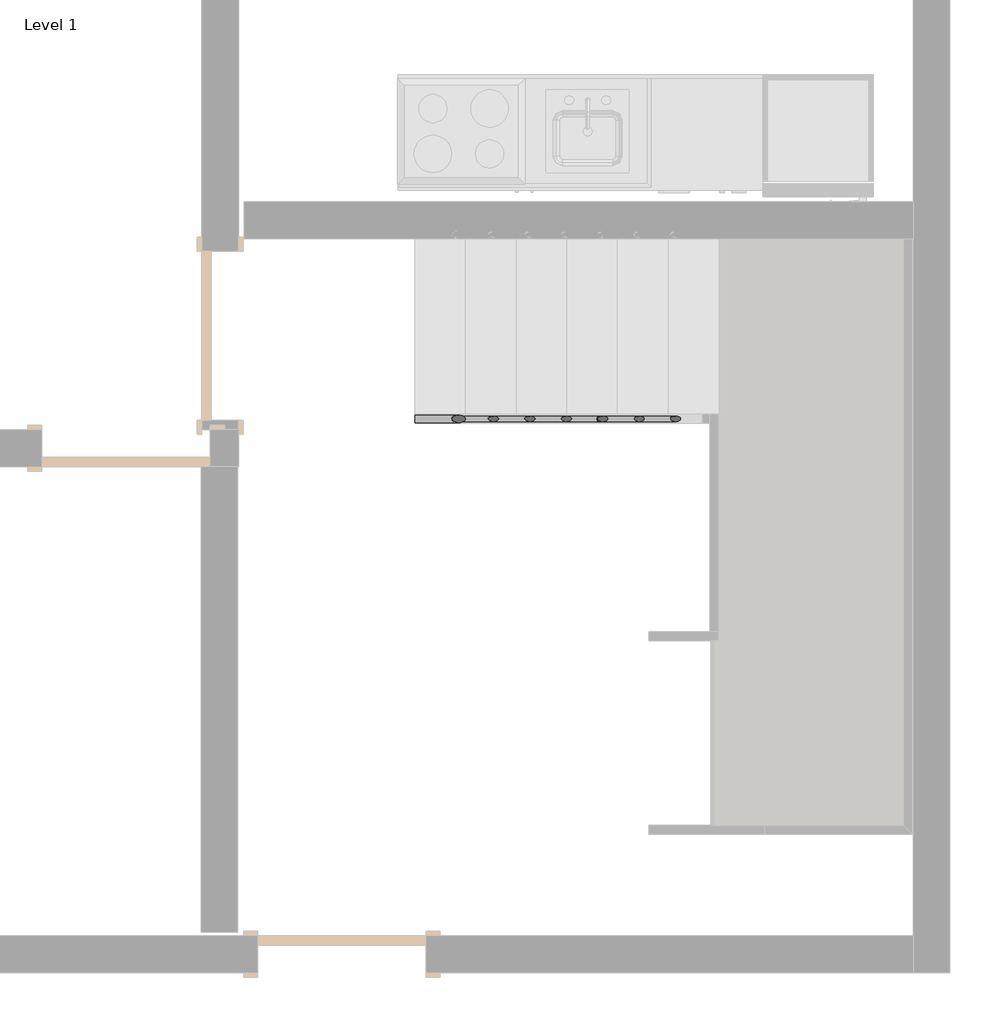
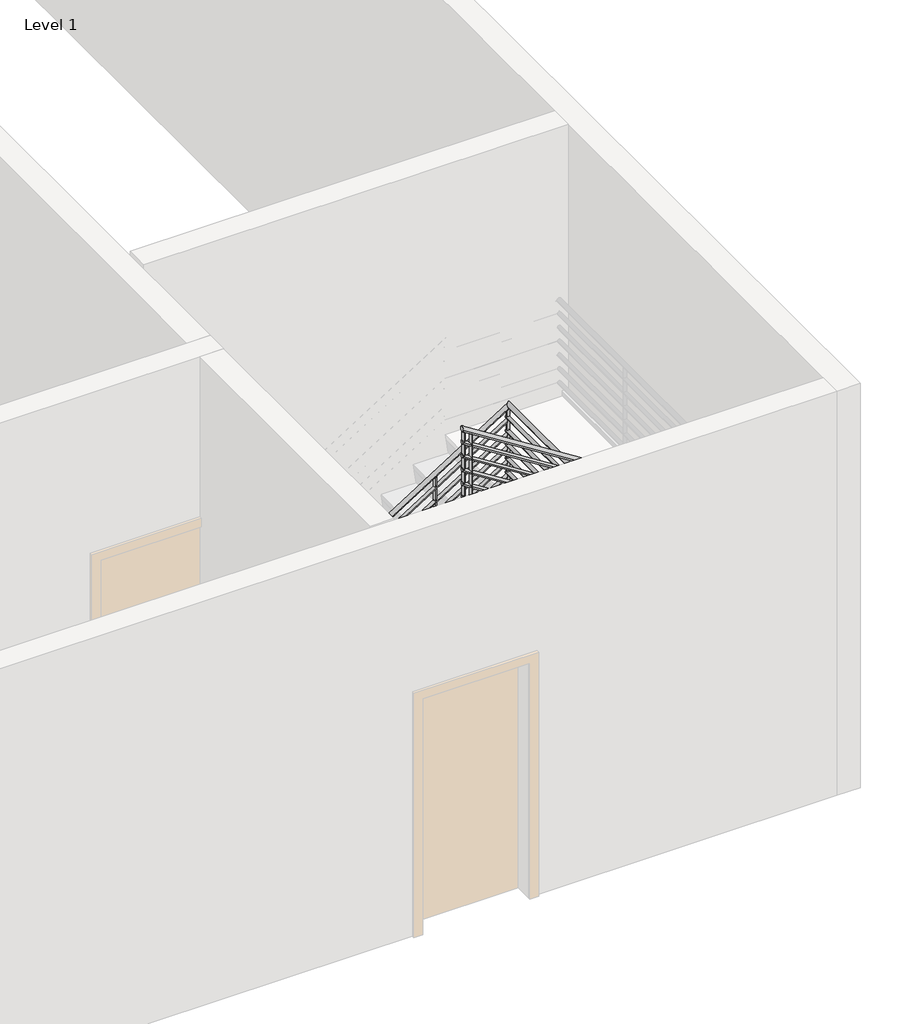
# One storey, part 2 of 4: 1 railing.
"""IFC4 building model written with IfcOpenShell, lengths in millimetres."""

from ifc_helpers import new_model, si_unit, point, frame, frame_2d, origin, place, context, project, spatial, circle_curve, ellipse_curve, trimmed, segment, composite_curve, outline, extrude, element, save
from ifc_brep_helpers import plane_surface, cylinder_surface, advanced_brep

model = new_model("IFC4")

# Units and contexts
model_context = context("Model", 3, world=origin())
ifc_project = project(units=[si_unit("LENGTHUNIT", "METRE", prefix="MILLI")], contexts=[model_context])

# Site, building, storey
site = spatial("IfcSite", under=ifc_project)
building = spatial("IfcBuilding", under=site)
storey = spatial("IfcBuildingStorey", under=building, Name="Level 1", Elevation=0.0)

# Railing
placement = place(None, origin())
element("IfcRailing", 1, ObjectType="900mm Pipe", at=placement, inside=storey, context=model_context, shape_type="SolidModel", body=[
    advanced_brep(
    [(-8739.5726707, 1114.9053702, 1050.2491997), (-8739.5726707, 1154.9053702, 1050.2491997), (-7121.1861826, 1114.9053702, 2073.7347258), (-7087.3793333, 1154.9053702, 2095.1145514)],
    [
        (0, 1, ellipse_curve(frame((-8739.5726707, 1134.9053702, 1050.2491997), z_axis=(-1.0, 0.0, 0.0), x_axis=(0.0, 0.0, -1.0)), 23.6638438, 20.0)),
        (1, 0, ellipse_curve(frame((-8739.5726707, 1134.9053702, 1050.2491997), z_axis=(-1.0, 0.0, 0.0), x_axis=(0.0, 0.0, -1.0)), 23.6638438, 20.0)),
        (2, 3, ellipse_curve(frame((-7104.2827579, 1134.9053702, 2084.4246386), z_axis=(0.5976263089853383, -0.7071067811865501, 0.37794549184843773), x_axis=(-0.5976263089853444, -0.7071067811865451, -0.37794549184843684)), 28.2842712, 20.0)),
        (3, 2, ellipse_curve(frame((-7104.2827579, 1134.9053702, 2084.4246386), z_axis=(0.5976263089853383, -0.7071067811865501, 0.37794549184843773), x_axis=(-0.5976263089853444, -0.7071067811865451, -0.37794549184843684)), 28.2842712, 20.0)),
        (0, 2),
        (3, 1),
    ],
    [
        plane_surface(frame((-8739.5726707, 1134.9053702, 1073.9130435), z_axis=(-1.0, 0.0, 0.0), x_axis=(0.0, 1.0, 0.0))),
        plane_surface(frame((-7114.9726707, 1134.9053702, 2101.3280632), z_axis=(0.5976263089853383, -0.7071067811865501, 0.37794549184843773), x_axis=(0.80177477810702, 0.527062745346942, -0.28171273961037624))),
        cylinder_surface(frame((-8728.8827579, 1134.9053702, 1057.0096189), z_axis=(-0.8451712313980437, 0.0, -0.5344956404098301), x_axis=(0.0, 1.0, 0.0)), 20.0),
    ],
    [
        (0, [[1, 2]]),
        (1, [[3, 4]]),
        (2, [[-1, 5, -4, 6]]),
        (2, [[-2, -6, -3, -5]]),
    ],
),
    advanced_brep(
    [(-7134.9726707, 1107.3120327, 2097.3913043), (-7094.9726707, 1141.118882, 2097.3913043), (-7134.9726707, -43.6804955, 2097.3913043), (-7094.9726707, -43.6804955, 2097.3913043)],
    [
        (0, 1, ellipse_curve(frame((-7114.9726707, 1124.2154574, 2097.3913043), z_axis=(-0.5976263089853383, 0.7071067811865501, -0.37794549184843773), x_axis=(0.5976263089853447, 0.7071067811865448, 0.3779454918484371)), 28.2842712, 20.0)),
        (1, 0, ellipse_curve(frame((-7114.9726707, 1124.2154574, 2097.3913043), z_axis=(-0.5976263089853383, 0.7071067811865501, -0.37794549184843773), x_axis=(0.5976263089853447, 0.7071067811865448, 0.3779454918484371)), 28.2842712, 20.0)),
        (2, 3, ellipse_curve(frame((-7114.9726707, -43.6804955, 2097.3913043), z_axis=(0.0, -0.7071067811865477, 0.7071067811865474), x_axis=(0.0, 0.7071067811865474, 0.7071067811865477)), 28.2842712, 20.0)),
        (3, 2, ellipse_curve(frame((-7114.9726707, -43.6804955, 2097.3913043), z_axis=(0.0, -0.7071067811865477, 0.7071067811865474), x_axis=(0.0, 0.7071067811865474, 0.7071067811865477)), 28.2842712, 20.0)),
        (0, 2),
        (3, 1),
    ],
    [
        plane_surface(frame((-7114.9726707, 1134.9053702, 2117.3913043), z_axis=(-0.5976263089853383, 0.7071067811865501, -0.37794549184843773), x_axis=(0.80177477810702, 0.527062745346942, -0.28171273961037624))),
        plane_surface(frame((-7114.9726707, -23.6804955, 2117.3913043), z_axis=(0.0, -0.7071067811865477, 0.7071067811865474), x_axis=(1.0, 0.0, 0.0))),
        cylinder_surface(frame((-7114.9726707, 1134.9053702, 2097.3913043), z_axis=(0.0, 1.0, 0.0), x_axis=(1.0, 0.0, 0.0)), 20.0),
    ],
    [
        (0, [[1, 2]]),
        (1, [[3, 4]]),
        (2, [[-1, 5, -4, 6]]),
        (2, [[-2, -6, -3, -5]]),
    ],
),
    advanced_brep(
    [(-7114.9726707, -23.6804955, 2283.7037451), (-7114.9726707, -63.6804955, 2283.7037451), (-8189.5726707, -23.6804955, 2963.2926779), (-8189.5726707, -63.6804955, 2963.2926779)],
    [
        (0, 1, ellipse_curve(frame((-7114.9726707, -43.6804955, 2283.7037451), z_axis=(0.4824439654458172, 0.0, -0.8759268349610687), x_axis=(0.8759268349610684, 0.0, 0.48244396544581747)), 22.8329573, 20.0)),
        (1, 0, ellipse_curve(frame((-7114.9726707, -43.6804955, 2283.7037451), z_axis=(0.4824439654458172, 0.0, -0.8759268349610687), x_axis=(0.8759268349610684, 0.0, 0.48244396544581747)), 22.8329573, 20.0)),
        (2, 3, ellipse_curve(frame((-8189.5726707, -43.6804955, 2963.2926779), z_axis=(-1.0, 0.0, 0.0), x_axis=(0.0, 0.0, -1.0)), 23.6638438, 20.0)),
        (3, 2, ellipse_curve(frame((-8189.5726707, -43.6804955, 2963.2926779), z_axis=(-1.0, 0.0, 0.0), x_axis=(0.0, 0.0, -1.0)), 23.6638438, 20.0)),
        (0, 2),
        (3, 1),
    ],
    [
        plane_surface(frame((-7094.9726707, -43.6804955, 2294.7193676), z_axis=(0.4824439654458172, 0.0, -0.8759268349610687), x_axis=(0.8759268349610687, 0.0, 0.4824439654458172))),
        plane_surface(frame((-8189.5726707, -43.6804955, 2986.9565217), z_axis=(-1.0, 0.0, 0.0), x_axis=(0.0, -1.0, 0.0))),
        cylinder_surface(frame((-7105.6625835, -43.6804955, 2277.815943), z_axis=(0.8451712313980436, 0.0, -0.5344956404098304), x_axis=(0.0, -1.0, 0.0)), 20.0),
    ],
    [
        (0, [[1, 2]]),
        (1, [[3, 4]]),
        (2, [[-1, 5, -4, 6]]),
        (2, [[-2, -6, -3, -5]]),
    ],
),
    advanced_brep(
    [(-7134.9726707, -43.6804955, 2097.3913043), (-7094.9726707, -43.6804955, 2097.3913043), (-7134.9726707, -43.6804955, 2272.6881227), (-7094.9726707, -43.6804955, 2294.7193676)],
    [
        (0, 1, ellipse_curve(frame((-7114.9726707, -43.6804955, 2097.3913043), z_axis=(0.0, 0.7071067811865477, -0.7071067811865474), x_axis=(0.0, -0.7071067811865474, -0.7071067811865478)), 28.2842712, 20.0)),
        (1, 0, ellipse_curve(frame((-7114.9726707, -43.6804955, 2097.3913043), z_axis=(0.0, 0.7071067811865477, -0.7071067811865474), x_axis=(0.0, -0.7071067811865474, -0.7071067811865478)), 28.2842712, 20.0)),
        (2, 3, ellipse_curve(frame((-7114.9726707, -43.6804955, 2283.7037451), z_axis=(-0.4824439654458172, 0.0, 0.8759268349610687), x_axis=(-0.8759268349610689, 0.0, -0.4824439654458169)), 22.8329573, 20.0)),
        (3, 2, ellipse_curve(frame((-7114.9726707, -43.6804955, 2283.7037451), z_axis=(-0.4824439654458172, 0.0, 0.8759268349610687), x_axis=(-0.8759268349610689, 0.0, -0.4824439654458169)), 22.8329573, 20.0)),
        (0, 2),
        (3, 1),
    ],
    [
        plane_surface(frame((-7114.9726707, -43.6804955, 2097.3913043), z_axis=(0.0, 0.7071067811865477, -0.7071067811865474), x_axis=(1.0, 0.0, 0.0))),
        plane_surface(frame((-7114.9726707, -43.6804955, 2283.7037451), z_axis=(-0.4824439654458172, 0.0, 0.8759268349610687), x_axis=(0.8759268349610687, 0.0, 0.4824439654458172))),
        cylinder_surface(frame((-7114.9726707, -43.6804955, 2097.3913043), z_axis=(0.0, 0.0, -1.0), x_axis=(1.0, 0.0, 0.0)), 20.0),
    ],
    [
        (0, [[1, 2]]),
        (1, [[3, 4]]),
        (2, [[-1, 5, -4, 6]]),
        (2, [[-2, -6, -3, -5]]),
    ],
),
    advanced_brep(
    [(-8739.5726707, 1119.9053702, 931.1651606), (-8739.5726707, 1149.9053702, 931.1651606), (-7129.9726707, 1119.9053702, 1949.0940144), (-7129.9726707, 1149.9053702, 1949.0940144)],
    [
        (0, 1, ellipse_curve(frame((-8739.5726707, 1134.9053702, 931.1651606), z_axis=(-1.0, 0.0, 0.0), x_axis=(0.0, 0.0, -1.0)), 17.7478828, 15.0)),
        (1, 0, ellipse_curve(frame((-8739.5726707, 1134.9053702, 931.1651606), z_axis=(-1.0, 0.0, 0.0), x_axis=(0.0, 0.0, -1.0)), 17.7478828, 15.0)),
        (2, 3, ellipse_curve(frame((-7129.9726707, 1134.9053702, 1949.0940144), z_axis=(1.0, 0.0, 0.0), x_axis=(0.0, 0.0, -1.0)), 17.7478828, 15.0)),
        (3, 2, ellipse_curve(frame((-7129.9726707, 1134.9053702, 1949.0940144), z_axis=(1.0, 0.0, 0.0), x_axis=(0.0, 0.0, -1.0)), 17.7478828, 15.0)),
        (1, 3),
        (2, 0),
    ],
    [
        plane_surface(frame((-8739.5726707, 1134.9053702, 948.9130435), z_axis=(-1.0, 0.0, 0.0), x_axis=(0.0, 1.0, 0.0))),
        plane_surface(frame((-7129.9726707, 1134.9053702, 1966.8418972), z_axis=(1.0, 0.0, 0.0), x_axis=(0.0, 1.0, 0.0))),
        cylinder_surface(frame((-8731.5552361, 1134.9053702, 936.235475), z_axis=(-0.8451712313980437, 0.0, -0.5344956404098302), x_axis=(0.0, 1.0, 0.0)), 15.0),
    ],
    [
        (0, [[1, 2]]),
        (1, [[3, 4]]),
        (2, [[-2, 5, -3, 6]]),
        (2, [[-1, -6, -4, -5]]),
    ],
),
    advanced_brep(
    [(-7129.9726707, 1149.9053702, 1977.3913043), (-7099.9726707, 1149.9053702, 1977.3913043), (-7129.9726707, -28.6804955, 1977.3913043), (-7099.9726707, -28.6804955, 1977.3913043)],
    [
        (0, 1, circle_curve(frame((-7114.9726707, 1149.9053702, 1977.3913043), z_axis=(0.0, 1.0, 0.0), x_axis=(1.0, 0.0, 0.0)), 15.0)),
        (1, 0, circle_curve(frame((-7114.9726707, 1149.9053702, 1977.3913043), z_axis=(0.0, 1.0, 0.0), x_axis=(1.0, 0.0, 0.0)), 15.0)),
        (2, 3, circle_curve(frame((-7114.9726707, -28.6804955, 1977.3913043), z_axis=(0.0, -1.0, 0.0), x_axis=(1.0, 0.0, 0.0)), 15.0)),
        (3, 2, circle_curve(frame((-7114.9726707, -28.6804955, 1977.3913043), z_axis=(0.0, -1.0, 0.0), x_axis=(1.0, 0.0, 0.0)), 15.0)),
        (1, 3),
        (2, 0),
    ],
    [
        plane_surface(frame((-7114.9726707, 1149.9053702, 1992.3913043), z_axis=(0.0, 1.0, 0.0), x_axis=(0.0, 0.0, -1.0))),
        plane_surface(frame((-7114.9726707, -28.6804955, 1992.3913043), z_axis=(0.0, -1.0, 0.0), x_axis=(0.0, 0.0, -1.0))),
        cylinder_surface(frame((-7114.9726707, 1149.9053702, 1977.3913043), z_axis=(0.0, 1.0, 0.0), x_axis=(1.0, 0.0, 0.0)), 15.0),
    ],
    [
        (0, [[1, 2]]),
        (1, [[3, 4]]),
        (2, [[-2, 5, -3, 6]]),
        (2, [[-1, -6, -4, -5]]),
    ],
),
    advanced_brep(
    [(-7099.9726707, -28.6804955, 2155.1335401), (-7099.9726707, -58.6804955, 2155.1335401), (-8189.5726707, -28.6804955, 2844.2086389), (-8189.5726707, -58.6804955, 2844.2086389)],
    [
        (0, 1, ellipse_curve(frame((-7099.9726707, -43.6804955, 2155.1335401), z_axis=(1.0, 0.0, 0.0), x_axis=(0.0, 0.0, -1.0)), 17.7478828, 15.0)),
        (1, 0, ellipse_curve(frame((-7099.9726707, -43.6804955, 2155.1335401), z_axis=(1.0, 0.0, 0.0), x_axis=(0.0, 0.0, -1.0)), 17.7478828, 15.0)),
        (2, 3, ellipse_curve(frame((-8189.5726707, -43.6804955, 2844.2086389), z_axis=(-1.0, 0.0, 0.0), x_axis=(0.0, 0.0, -1.0)), 17.7478828, 15.0)),
        (3, 2, ellipse_curve(frame((-8189.5726707, -43.6804955, 2844.2086389), z_axis=(-1.0, 0.0, 0.0), x_axis=(0.0, 0.0, -1.0)), 17.7478828, 15.0)),
        (1, 3),
        (2, 0),
    ],
    [
        plane_surface(frame((-7099.9726707, -43.6804955, 2172.8814229), z_axis=(1.0, 0.0, 0.0), x_axis=(0.0, -1.0, 0.0))),
        plane_surface(frame((-8189.5726707, -43.6804955, 2861.9565217), z_axis=(-1.0, 0.0, 0.0), x_axis=(0.0, -1.0, 0.0))),
        cylinder_surface(frame((-7107.9901053, -43.6804955, 2160.2038545), z_axis=(0.8451712313980437, 0.0, -0.5344956404098303), x_axis=(0.0, -1.0, 0.0)), 15.0),
    ],
    [
        (0, [[1, 2]]),
        (1, [[3, 4]]),
        (2, [[-2, 5, -3, 6]]),
        (2, [[-1, -6, -4, -5]]),
    ],
),
    advanced_brep(
    [(-8739.5726707, 1119.9053702, 806.1651606), (-8739.5726707, 1149.9053702, 806.1651606), (-7129.9726707, 1119.9053702, 1824.0940144), (-7129.9726707, 1149.9053702, 1824.0940144)],
    [
        (0, 1, ellipse_curve(frame((-8739.5726707, 1134.9053702, 806.1651606), z_axis=(-1.0, 0.0, 0.0), x_axis=(0.0, 0.0, -1.0)), 17.7478828, 15.0)),
        (1, 0, ellipse_curve(frame((-8739.5726707, 1134.9053702, 806.1651606), z_axis=(-1.0, 0.0, 0.0), x_axis=(0.0, 0.0, -1.0)), 17.7478828, 15.0)),
        (2, 3, ellipse_curve(frame((-7129.9726707, 1134.9053702, 1824.0940144), z_axis=(1.0, 0.0, 0.0), x_axis=(0.0, 0.0, -1.0)), 17.7478828, 15.0)),
        (3, 2, ellipse_curve(frame((-7129.9726707, 1134.9053702, 1824.0940144), z_axis=(1.0, 0.0, 0.0), x_axis=(0.0, 0.0, -1.0)), 17.7478828, 15.0)),
        (1, 3),
        (2, 0),
    ],
    [
        plane_surface(frame((-8739.5726707, 1134.9053702, 823.9130435), z_axis=(-1.0, 0.0, 0.0), x_axis=(0.0, 1.0, 0.0))),
        plane_surface(frame((-7129.9726707, 1134.9053702, 1841.8418972), z_axis=(1.0, 0.0, 0.0), x_axis=(0.0, 1.0, 0.0))),
        cylinder_surface(frame((-8731.5552361, 1134.9053702, 811.235475), z_axis=(-0.8451712313980438, 0.0, -0.5344956404098301), x_axis=(0.0, 1.0, 0.0)), 15.0),
    ],
    [
        (0, [[1, 2]]),
        (1, [[3, 4]]),
        (2, [[-2, 5, -3, 6]]),
        (2, [[-1, -6, -4, -5]]),
    ],
),
    advanced_brep(
    [(-7129.9726707, 1149.9053702, 1852.3913043), (-7099.9726707, 1149.9053702, 1852.3913043), (-7129.9726707, -28.6804955, 1852.3913043), (-7099.9726707, -28.6804955, 1852.3913043)],
    [
        (0, 1, circle_curve(frame((-7114.9726707, 1149.9053702, 1852.3913043), z_axis=(0.0, 1.0, 0.0), x_axis=(1.0, 0.0, 0.0)), 15.0)),
        (1, 0, circle_curve(frame((-7114.9726707, 1149.9053702, 1852.3913043), z_axis=(0.0, 1.0, 0.0), x_axis=(1.0, 0.0, 0.0)), 15.0)),
        (2, 3, circle_curve(frame((-7114.9726707, -28.6804955, 1852.3913043), z_axis=(0.0, -1.0, 0.0), x_axis=(1.0, 0.0, 0.0)), 15.0)),
        (3, 2, circle_curve(frame((-7114.9726707, -28.6804955, 1852.3913043), z_axis=(0.0, -1.0, 0.0), x_axis=(1.0, 0.0, 0.0)), 15.0)),
        (1, 3),
        (2, 0),
    ],
    [
        plane_surface(frame((-7114.9726707, 1149.9053702, 1867.3913043), z_axis=(0.0, 1.0, 0.0), x_axis=(0.0, 0.0, -1.0))),
        plane_surface(frame((-7114.9726707, -28.6804955, 1867.3913043), z_axis=(0.0, -1.0, 0.0), x_axis=(0.0, 0.0, -1.0))),
        cylinder_surface(frame((-7114.9726707, 1149.9053702, 1852.3913043), z_axis=(0.0, 1.0, 0.0), x_axis=(1.0, 0.0, 0.0)), 15.0),
    ],
    [
        (0, [[1, 2]]),
        (1, [[3, 4]]),
        (2, [[-2, 5, -3, 6]]),
        (2, [[-1, -6, -4, -5]]),
    ],
),
    advanced_brep(
    [(-7099.9726707, -28.6804955, 2030.1335401), (-7099.9726707, -58.6804955, 2030.1335401), (-8189.5726707, -28.6804955, 2719.2086389), (-8189.5726707, -58.6804955, 2719.2086389)],
    [
        (0, 1, ellipse_curve(frame((-7099.9726707, -43.6804955, 2030.1335401), z_axis=(1.0, 0.0, 0.0), x_axis=(0.0, 0.0, -1.0)), 17.7478828, 15.0)),
        (1, 0, ellipse_curve(frame((-7099.9726707, -43.6804955, 2030.1335401), z_axis=(1.0, 0.0, 0.0), x_axis=(0.0, 0.0, -1.0)), 17.7478828, 15.0)),
        (2, 3, ellipse_curve(frame((-8189.5726707, -43.6804955, 2719.2086389), z_axis=(-1.0, 0.0, 0.0), x_axis=(0.0, 0.0, -1.0)), 17.7478828, 15.0)),
        (3, 2, ellipse_curve(frame((-8189.5726707, -43.6804955, 2719.2086389), z_axis=(-1.0, 0.0, 0.0), x_axis=(0.0, 0.0, -1.0)), 17.7478828, 15.0)),
        (1, 3),
        (2, 0),
    ],
    [
        plane_surface(frame((-7099.9726707, -43.6804955, 2047.8814229), z_axis=(1.0, 0.0, 0.0), x_axis=(0.0, -1.0, 0.0))),
        plane_surface(frame((-8189.5726707, -43.6804955, 2736.9565217), z_axis=(-1.0, 0.0, 0.0), x_axis=(0.0, -1.0, 0.0))),
        cylinder_surface(frame((-7107.9901053, -43.6804955, 2035.2038545), z_axis=(0.8451712313980436, 0.0, -0.5344956404098304), x_axis=(0.0, -1.0, 0.0)), 15.0),
    ],
    [
        (0, [[1, 2]]),
        (1, [[3, 4]]),
        (2, [[-2, 5, -3, 6]]),
        (2, [[-1, -6, -4, -5]]),
    ],
),
    advanced_brep(
    [(-8739.5726707, 1119.9053702, 681.1651606), (-8739.5726707, 1149.9053702, 681.1651606), (-7129.9726707, 1119.9053702, 1699.0940144), (-7129.9726707, 1149.9053702, 1699.0940144)],
    [
        (0, 1, ellipse_curve(frame((-8739.5726707, 1134.9053702, 681.1651606), z_axis=(-1.0, 0.0, 0.0), x_axis=(0.0, 0.0, -1.0)), 17.7478828, 15.0)),
        (1, 0, ellipse_curve(frame((-8739.5726707, 1134.9053702, 681.1651606), z_axis=(-1.0, 0.0, 0.0), x_axis=(0.0, 0.0, -1.0)), 17.7478828, 15.0)),
        (2, 3, ellipse_curve(frame((-7129.9726707, 1134.9053702, 1699.0940144), z_axis=(1.0, 0.0, 0.0), x_axis=(0.0, 0.0, -1.0)), 17.7478828, 15.0)),
        (3, 2, ellipse_curve(frame((-7129.9726707, 1134.9053702, 1699.0940144), z_axis=(1.0, 0.0, 0.0), x_axis=(0.0, 0.0, -1.0)), 17.7478828, 15.0)),
        (1, 3),
        (2, 0),
    ],
    [
        plane_surface(frame((-8739.5726707, 1134.9053702, 698.9130435), z_axis=(-1.0, 0.0, 0.0), x_axis=(0.0, 1.0, 0.0))),
        plane_surface(frame((-7129.9726707, 1134.9053702, 1716.8418972), z_axis=(1.0, 0.0, 0.0), x_axis=(0.0, 1.0, 0.0))),
        cylinder_surface(frame((-8731.5552361, 1134.9053702, 686.235475), z_axis=(-0.8451712313980437, 0.0, -0.5344956404098302), x_axis=(0.0, 1.0, 0.0)), 15.0),
    ],
    [
        (0, [[1, 2]]),
        (1, [[3, 4]]),
        (2, [[-2, 5, -3, 6]]),
        (2, [[-1, -6, -4, -5]]),
    ],
),
    advanced_brep(
    [(-7129.9726707, 1149.9053702, 1727.3913043), (-7099.9726707, 1149.9053702, 1727.3913043), (-7129.9726707, -28.6804955, 1727.3913043), (-7099.9726707, -28.6804955, 1727.3913043)],
    [
        (0, 1, circle_curve(frame((-7114.9726707, 1149.9053702, 1727.3913043), z_axis=(0.0, 1.0, 0.0), x_axis=(1.0, 0.0, 0.0)), 15.0)),
        (1, 0, circle_curve(frame((-7114.9726707, 1149.9053702, 1727.3913043), z_axis=(0.0, 1.0, 0.0), x_axis=(1.0, 0.0, 0.0)), 15.0)),
        (2, 3, circle_curve(frame((-7114.9726707, -28.6804955, 1727.3913043), z_axis=(0.0, -1.0, 0.0), x_axis=(1.0, 0.0, 0.0)), 15.0)),
        (3, 2, circle_curve(frame((-7114.9726707, -28.6804955, 1727.3913043), z_axis=(0.0, -1.0, 0.0), x_axis=(1.0, 0.0, 0.0)), 15.0)),
        (1, 3),
        (2, 0),
    ],
    [
        plane_surface(frame((-7114.9726707, 1149.9053702, 1742.3913043), z_axis=(0.0, 1.0, 0.0), x_axis=(0.0, 0.0, -1.0))),
        plane_surface(frame((-7114.9726707, -28.6804955, 1742.3913043), z_axis=(0.0, -1.0, 0.0), x_axis=(0.0, 0.0, -1.0))),
        cylinder_surface(frame((-7114.9726707, 1149.9053702, 1727.3913043), z_axis=(0.0, 1.0, 0.0), x_axis=(1.0, 0.0, 0.0)), 15.0),
    ],
    [
        (0, [[1, 2]]),
        (1, [[3, 4]]),
        (2, [[-2, 5, -3, 6]]),
        (2, [[-1, -6, -4, -5]]),
    ],
),
    advanced_brep(
    [(-7099.9726707, -28.6804955, 1905.1335401), (-7099.9726707, -58.6804955, 1905.1335401), (-8189.5726707, -28.6804955, 2594.2086389), (-8189.5726707, -58.6804955, 2594.2086389)],
    [
        (0, 1, ellipse_curve(frame((-7099.9726707, -43.6804955, 1905.1335401), z_axis=(1.0, 0.0, 0.0), x_axis=(0.0, 0.0, -1.0)), 17.7478828, 15.0)),
        (1, 0, ellipse_curve(frame((-7099.9726707, -43.6804955, 1905.1335401), z_axis=(1.0, 0.0, 0.0), x_axis=(0.0, 0.0, -1.0)), 17.7478828, 15.0)),
        (2, 3, ellipse_curve(frame((-8189.5726707, -43.6804955, 2594.2086389), z_axis=(-1.0, 0.0, 0.0), x_axis=(0.0, 0.0, -1.0)), 17.7478828, 15.0)),
        (3, 2, ellipse_curve(frame((-8189.5726707, -43.6804955, 2594.2086389), z_axis=(-1.0, 0.0, 0.0), x_axis=(0.0, 0.0, -1.0)), 17.7478828, 15.0)),
        (1, 3),
        (2, 0),
    ],
    [
        plane_surface(frame((-7099.9726707, -43.6804955, 1922.8814229), z_axis=(1.0, 0.0, 0.0), x_axis=(0.0, -1.0, 0.0))),
        plane_surface(frame((-8189.5726707, -43.6804955, 2611.9565217), z_axis=(-1.0, 0.0, 0.0), x_axis=(0.0, -1.0, 0.0))),
        cylinder_surface(frame((-7107.9901053, -43.6804955, 1910.2038545), z_axis=(0.8451712313980435, 0.0, -0.5344956404098306), x_axis=(0.0, -1.0, 0.0)), 15.0),
    ],
    [
        (0, [[1, 2]]),
        (1, [[3, 4]]),
        (2, [[-2, 5, -3, 6]]),
        (2, [[-1, -6, -4, -5]]),
    ],
),
    advanced_brep(
    [(-8739.5726707, 1119.9053702, 556.1651606), (-8739.5726707, 1149.9053702, 556.1651606), (-7129.9726707, 1119.9053702, 1574.0940144), (-7129.9726707, 1149.9053702, 1574.0940144)],
    [
        (0, 1, ellipse_curve(frame((-8739.5726707, 1134.9053702, 556.1651606), z_axis=(-1.0, 0.0, 0.0), x_axis=(0.0, 0.0, -1.0)), 17.7478828, 15.0)),
        (1, 0, ellipse_curve(frame((-8739.5726707, 1134.9053702, 556.1651606), z_axis=(-1.0, 0.0, 0.0), x_axis=(0.0, 0.0, -1.0)), 17.7478828, 15.0)),
        (2, 3, ellipse_curve(frame((-7129.9726707, 1134.9053702, 1574.0940144), z_axis=(1.0, 0.0, 0.0), x_axis=(0.0, 0.0, -1.0)), 17.7478828, 15.0)),
        (3, 2, ellipse_curve(frame((-7129.9726707, 1134.9053702, 1574.0940144), z_axis=(1.0, 0.0, 0.0), x_axis=(0.0, 0.0, -1.0)), 17.7478828, 15.0)),
        (1, 3),
        (2, 0),
    ],
    [
        plane_surface(frame((-8739.5726707, 1134.9053702, 573.9130435), z_axis=(-1.0, 0.0, 0.0), x_axis=(0.0, 1.0, 0.0))),
        plane_surface(frame((-7129.9726707, 1134.9053702, 1591.8418972), z_axis=(1.0, 0.0, 0.0), x_axis=(0.0, 1.0, 0.0))),
        cylinder_surface(frame((-8731.5552361, 1134.9053702, 561.235475), z_axis=(-0.8451712313980438, 0.0, -0.5344956404098301), x_axis=(0.0, 1.0, 0.0)), 15.0),
    ],
    [
        (0, [[1, 2]]),
        (1, [[3, 4]]),
        (2, [[-2, 5, -3, 6]]),
        (2, [[-1, -6, -4, -5]]),
    ],
),
    advanced_brep(
    [(-7129.9726707, 1149.9053702, 1602.3913043), (-7099.9726707, 1149.9053702, 1602.3913043), (-7129.9726707, -28.6804955, 1602.3913043), (-7099.9726707, -28.6804955, 1602.3913043)],
    [
        (0, 1, circle_curve(frame((-7114.9726707, 1149.9053702, 1602.3913043), z_axis=(0.0, 1.0, 0.0), x_axis=(1.0, 0.0, 0.0)), 15.0)),
        (1, 0, circle_curve(frame((-7114.9726707, 1149.9053702, 1602.3913043), z_axis=(0.0, 1.0, 0.0), x_axis=(1.0, 0.0, 0.0)), 15.0)),
        (2, 3, circle_curve(frame((-7114.9726707, -28.6804955, 1602.3913043), z_axis=(0.0, -1.0, 0.0), x_axis=(1.0, 0.0, 0.0)), 15.0)),
        (3, 2, circle_curve(frame((-7114.9726707, -28.6804955, 1602.3913043), z_axis=(0.0, -1.0, 0.0), x_axis=(1.0, 0.0, 0.0)), 15.0)),
        (1, 3),
        (2, 0),
    ],
    [
        plane_surface(frame((-7114.9726707, 1149.9053702, 1617.3913043), z_axis=(0.0, 1.0, 0.0), x_axis=(0.0, 0.0, -1.0))),
        plane_surface(frame((-7114.9726707, -28.6804955, 1617.3913043), z_axis=(0.0, -1.0, 0.0), x_axis=(0.0, 0.0, -1.0))),
        cylinder_surface(frame((-7114.9726707, 1149.9053702, 1602.3913043), z_axis=(0.0, 1.0, 0.0), x_axis=(1.0, 0.0, 0.0)), 15.0),
    ],
    [
        (0, [[1, 2]]),
        (1, [[3, 4]]),
        (2, [[-2, 5, -3, 6]]),
        (2, [[-1, -6, -4, -5]]),
    ],
),
    advanced_brep(
    [(-7099.9726707, -28.6804955, 1780.1335401), (-7099.9726707, -58.6804955, 1780.1335401), (-8189.5726707, -28.6804955, 2469.2086389), (-8189.5726707, -58.6804955, 2469.2086389)],
    [
        (0, 1, ellipse_curve(frame((-7099.9726707, -43.6804955, 1780.1335401), z_axis=(1.0, 0.0, 0.0), x_axis=(0.0, 0.0, -1.0)), 17.7478828, 15.0)),
        (1, 0, ellipse_curve(frame((-7099.9726707, -43.6804955, 1780.1335401), z_axis=(1.0, 0.0, 0.0), x_axis=(0.0, 0.0, -1.0)), 17.7478828, 15.0)),
        (2, 3, ellipse_curve(frame((-8189.5726707, -43.6804955, 2469.2086389), z_axis=(-1.0, 0.0, 0.0), x_axis=(0.0, 0.0, -1.0)), 17.7478828, 15.0)),
        (3, 2, ellipse_curve(frame((-8189.5726707, -43.6804955, 2469.2086389), z_axis=(-1.0, 0.0, 0.0), x_axis=(0.0, 0.0, -1.0)), 17.7478828, 15.0)),
        (1, 3),
        (2, 0),
    ],
    [
        plane_surface(frame((-7099.9726707, -43.6804955, 1797.8814229), z_axis=(1.0, 0.0, 0.0), x_axis=(0.0, -1.0, 0.0))),
        plane_surface(frame((-8189.5726707, -43.6804955, 2486.9565217), z_axis=(-1.0, 0.0, 0.0), x_axis=(0.0, -1.0, 0.0))),
        cylinder_surface(frame((-7107.9901053, -43.6804955, 1785.2038545), z_axis=(0.8451712313980436, 0.0, -0.5344956404098304), x_axis=(0.0, -1.0, 0.0)), 15.0),
    ],
    [
        (0, [[1, 2]]),
        (1, [[3, 4]]),
        (2, [[-2, 5, -3, 6]]),
        (2, [[-1, -6, -4, -5]]),
    ],
),
    advanced_brep(
    [(-8739.5726707, 1119.9053702, 431.1651606), (-8739.5726707, 1149.9053702, 431.1651606), (-7129.9726707, 1119.9053702, 1449.0940144), (-7129.9726707, 1149.9053702, 1449.0940144)],
    [
        (0, 1, ellipse_curve(frame((-8739.5726707, 1134.9053702, 431.1651606), z_axis=(-1.0, 0.0, 0.0), x_axis=(0.0, 0.0, -1.0)), 17.7478828, 15.0)),
        (1, 0, ellipse_curve(frame((-8739.5726707, 1134.9053702, 431.1651606), z_axis=(-1.0, 0.0, 0.0), x_axis=(0.0, 0.0, -1.0)), 17.7478828, 15.0)),
        (2, 3, ellipse_curve(frame((-7129.9726707, 1134.9053702, 1449.0940144), z_axis=(1.0, 0.0, 0.0), x_axis=(0.0, 0.0, -1.0)), 17.7478828, 15.0)),
        (3, 2, ellipse_curve(frame((-7129.9726707, 1134.9053702, 1449.0940144), z_axis=(1.0, 0.0, 0.0), x_axis=(0.0, 0.0, -1.0)), 17.7478828, 15.0)),
        (1, 3),
        (2, 0),
    ],
    [
        plane_surface(frame((-8739.5726707, 1134.9053702, 448.9130435), z_axis=(-1.0, 0.0, 0.0), x_axis=(0.0, 1.0, 0.0))),
        plane_surface(frame((-7129.9726707, 1134.9053702, 1466.8418972), z_axis=(1.0, 0.0, 0.0), x_axis=(0.0, 1.0, 0.0))),
        cylinder_surface(frame((-8731.5552361, 1134.9053702, 436.235475), z_axis=(-0.8451712313980437, 0.0, -0.5344956404098302), x_axis=(0.0, 1.0, 0.0)), 15.0),
    ],
    [
        (0, [[1, 2]]),
        (1, [[3, 4]]),
        (2, [[-2, 5, -3, 6]]),
        (2, [[-1, -6, -4, -5]]),
    ],
),
    advanced_brep(
    [(-7129.9726707, 1149.9053702, 1477.3913043), (-7099.9726707, 1149.9053702, 1477.3913043), (-7129.9726707, -28.6804955, 1477.3913043), (-7099.9726707, -28.6804955, 1477.3913043)],
    [
        (0, 1, circle_curve(frame((-7114.9726707, 1149.9053702, 1477.3913043), z_axis=(0.0, 1.0, 0.0), x_axis=(1.0, 0.0, 0.0)), 15.0)),
        (1, 0, circle_curve(frame((-7114.9726707, 1149.9053702, 1477.3913043), z_axis=(0.0, 1.0, 0.0), x_axis=(1.0, 0.0, 0.0)), 15.0)),
        (2, 3, circle_curve(frame((-7114.9726707, -28.6804955, 1477.3913043), z_axis=(0.0, -1.0, 0.0), x_axis=(1.0, 0.0, 0.0)), 15.0)),
        (3, 2, circle_curve(frame((-7114.9726707, -28.6804955, 1477.3913043), z_axis=(0.0, -1.0, 0.0), x_axis=(1.0, 0.0, 0.0)), 15.0)),
        (1, 3),
        (2, 0),
    ],
    [
        plane_surface(frame((-7114.9726707, 1149.9053702, 1492.3913043), z_axis=(0.0, 1.0, 0.0), x_axis=(0.0, 0.0, -1.0))),
        plane_surface(frame((-7114.9726707, -28.6804955, 1492.3913043), z_axis=(0.0, -1.0, 0.0), x_axis=(0.0, 0.0, -1.0))),
        cylinder_surface(frame((-7114.9726707, 1149.9053702, 1477.3913043), z_axis=(0.0, 1.0, 0.0), x_axis=(1.0, 0.0, 0.0)), 15.0),
    ],
    [
        (0, [[1, 2]]),
        (1, [[3, 4]]),
        (2, [[-2, 5, -3, 6]]),
        (2, [[-1, -6, -4, -5]]),
    ],
),
    advanced_brep(
    [(-7099.9726707, -28.6804955, 1655.1335401), (-7099.9726707, -58.6804955, 1655.1335401), (-8189.5726707, -28.6804955, 2344.2086389), (-8189.5726707, -58.6804955, 2344.2086389)],
    [
        (0, 1, ellipse_curve(frame((-7099.9726707, -43.6804955, 1655.1335401), z_axis=(1.0, 0.0, 0.0), x_axis=(0.0, 0.0, -1.0)), 17.7478828, 15.0)),
        (1, 0, ellipse_curve(frame((-7099.9726707, -43.6804955, 1655.1335401), z_axis=(1.0, 0.0, 0.0), x_axis=(0.0, 0.0, -1.0)), 17.7478828, 15.0)),
        (2, 3, ellipse_curve(frame((-8189.5726707, -43.6804955, 2344.2086389), z_axis=(-1.0, 0.0, 0.0), x_axis=(0.0, 0.0, -1.0)), 17.7478828, 15.0)),
        (3, 2, ellipse_curve(frame((-8189.5726707, -43.6804955, 2344.2086389), z_axis=(-1.0, 0.0, 0.0), x_axis=(0.0, 0.0, -1.0)), 17.7478828, 15.0)),
        (1, 3),
        (2, 0),
    ],
    [
        plane_surface(frame((-7099.9726707, -43.6804955, 1672.8814229), z_axis=(1.0, 0.0, 0.0), x_axis=(0.0, -1.0, 0.0))),
        plane_surface(frame((-8189.5726707, -43.6804955, 2361.9565217), z_axis=(-1.0, 0.0, 0.0), x_axis=(0.0, -1.0, 0.0))),
        cylinder_surface(frame((-7107.9901053, -43.6804955, 1660.2038545), z_axis=(0.8451712313980436, 0.0, -0.5344956404098304), x_axis=(0.0, -1.0, 0.0)), 15.0),
    ],
    [
        (0, [[1, 2]]),
        (1, [[3, 4]]),
        (2, [[-2, 5, -3, 6]]),
        (2, [[-1, -6, -4, -5]]),
    ],
),
    advanced_brep(
    [(-8739.5726707, 1119.9053702, 306.1651606), (-8739.5726707, 1149.9053702, 306.1651606), (-7129.9726707, 1119.9053702, 1324.0940144), (-7129.9726707, 1149.9053702, 1324.0940144)],
    [
        (0, 1, ellipse_curve(frame((-8739.5726707, 1134.9053702, 306.1651606), z_axis=(-1.0, 0.0, 0.0), x_axis=(0.0, 0.0, -1.0)), 17.7478828, 15.0)),
        (1, 0, ellipse_curve(frame((-8739.5726707, 1134.9053702, 306.1651606), z_axis=(-1.0, 0.0, 0.0), x_axis=(0.0, 0.0, -1.0)), 17.7478828, 15.0)),
        (2, 3, ellipse_curve(frame((-7129.9726707, 1134.9053702, 1324.0940144), z_axis=(1.0, 0.0, 0.0), x_axis=(0.0, 0.0, -1.0)), 17.7478828, 15.0)),
        (3, 2, ellipse_curve(frame((-7129.9726707, 1134.9053702, 1324.0940144), z_axis=(1.0, 0.0, 0.0), x_axis=(0.0, 0.0, -1.0)), 17.7478828, 15.0)),
        (1, 3),
        (2, 0),
    ],
    [
        plane_surface(frame((-8739.5726707, 1134.9053702, 323.9130435), z_axis=(-1.0, 0.0, 0.0), x_axis=(0.0, 1.0, 0.0))),
        plane_surface(frame((-7129.9726707, 1134.9053702, 1341.8418972), z_axis=(1.0, 0.0, 0.0), x_axis=(0.0, 1.0, 0.0))),
        cylinder_surface(frame((-8731.5552361, 1134.9053702, 311.235475), z_axis=(-0.8451712313980438, 0.0, -0.5344956404098301), x_axis=(0.0, 1.0, 0.0)), 15.0),
    ],
    [
        (0, [[1, 2]]),
        (1, [[3, 4]]),
        (2, [[-2, 5, -3, 6]]),
        (2, [[-1, -6, -4, -5]]),
    ],
),
    advanced_brep(
    [(-7129.9726707, 1149.9053702, 1352.3913043), (-7099.9726707, 1149.9053702, 1352.3913043), (-7129.9726707, -28.6804955, 1352.3913043), (-7099.9726707, -28.6804955, 1352.3913043)],
    [
        (0, 1, circle_curve(frame((-7114.9726707, 1149.9053702, 1352.3913043), z_axis=(0.0, 1.0, 0.0), x_axis=(1.0, 0.0, 0.0)), 15.0)),
        (1, 0, circle_curve(frame((-7114.9726707, 1149.9053702, 1352.3913043), z_axis=(0.0, 1.0, 0.0), x_axis=(1.0, 0.0, 0.0)), 15.0)),
        (2, 3, circle_curve(frame((-7114.9726707, -28.6804955, 1352.3913043), z_axis=(0.0, -1.0, 0.0), x_axis=(1.0, 0.0, 0.0)), 15.0)),
        (3, 2, circle_curve(frame((-7114.9726707, -28.6804955, 1352.3913043), z_axis=(0.0, -1.0, 0.0), x_axis=(1.0, 0.0, 0.0)), 15.0)),
        (1, 3),
        (2, 0),
    ],
    [
        plane_surface(frame((-7114.9726707, 1149.9053702, 1367.3913043), z_axis=(0.0, 1.0, 0.0), x_axis=(0.0, 0.0, -1.0))),
        plane_surface(frame((-7114.9726707, -28.6804955, 1367.3913043), z_axis=(0.0, -1.0, 0.0), x_axis=(0.0, 0.0, -1.0))),
        cylinder_surface(frame((-7114.9726707, 1149.9053702, 1352.3913043), z_axis=(0.0, 1.0, 0.0), x_axis=(1.0, 0.0, 0.0)), 15.0),
    ],
    [
        (0, [[1, 2]]),
        (1, [[3, 4]]),
        (2, [[-2, 5, -3, 6]]),
        (2, [[-1, -6, -4, -5]]),
    ],
),
    advanced_brep(
    [(-7099.9726707, -28.6804955, 1530.1335401), (-7099.9726707, -58.6804955, 1530.1335401), (-8189.5726707, -28.6804955, 2219.2086389), (-8189.5726707, -58.6804955, 2219.2086389)],
    [
        (0, 1, ellipse_curve(frame((-7099.9726707, -43.6804955, 1530.1335401), z_axis=(1.0, 0.0, 0.0), x_axis=(0.0, 0.0, -1.0)), 17.7478828, 15.0)),
        (1, 0, ellipse_curve(frame((-7099.9726707, -43.6804955, 1530.1335401), z_axis=(1.0, 0.0, 0.0), x_axis=(0.0, 0.0, -1.0)), 17.7478828, 15.0)),
        (2, 3, ellipse_curve(frame((-8189.5726707, -43.6804955, 2219.2086389), z_axis=(-1.0, 0.0, 0.0), x_axis=(0.0, 0.0, -1.0)), 17.7478828, 15.0)),
        (3, 2, ellipse_curve(frame((-8189.5726707, -43.6804955, 2219.2086389), z_axis=(-1.0, 0.0, 0.0), x_axis=(0.0, 0.0, -1.0)), 17.7478828, 15.0)),
        (1, 3),
        (2, 0),
    ],
    [
        plane_surface(frame((-7099.9726707, -43.6804955, 1547.8814229), z_axis=(1.0, 0.0, 0.0), x_axis=(0.0, -1.0, 0.0))),
        plane_surface(frame((-8189.5726707, -43.6804955, 2236.9565217), z_axis=(-1.0, 0.0, 0.0), x_axis=(0.0, -1.0, 0.0))),
        cylinder_surface(frame((-7107.9901053, -43.6804955, 1535.2038545), z_axis=(0.8451712313980436, 0.0, -0.5344956404098304), x_axis=(0.0, -1.0, 0.0)), 15.0),
    ],
    [
        (0, [[1, 2]]),
        (1, [[3, 4]]),
        (2, [[-2, 5, -3, 6]]),
        (2, [[-1, -6, -4, -5]]),
    ],
),
    advanced_brep(
    [(-8114.9726707, -56.1804955, 2892.4509685), (-8114.9726707, -31.1804955, 2892.4509685), (-8114.9726707, -31.1804955, 2080.9551476), (-8114.9726707, -56.1804955, 2080.9551476)],
    [
        (0, 1, ellipse_curve(frame((-8114.9726707, -43.6804955, 2892.4509685), z_axis=(-0.5344956404098302, 0.0, -0.8451712313980437), x_axis=(-0.8451712313980437, 0.0, 0.53449564040983)), 14.7899024, 12.5)),
        (1, 2),
        (2, 3, ellipse_curve(frame((-8114.9726707, -43.6804955, 2080.9551476), z_axis=(0.5344956404098296, 0.0, 0.8451712313980442), x_axis=(-0.8451712313980442, 0.0, 0.5344956404098292)), 14.7899024, 12.5)),
        (3, 0),
        (3, 2, ellipse_curve(frame((-8114.9726707, -43.6804955, 2080.9551476), z_axis=(0.5344956404098296, 0.0, 0.8451712313980442), x_axis=(-0.8451712313980442, 0.0, 0.5344956404098292)), 14.7899024, 12.5)),
        (1, 0, ellipse_curve(frame((-8114.9726707, -43.6804955, 2892.4509685), z_axis=(-0.5344956404098302, 0.0, -0.8451712313980437), x_axis=(-0.8451712313980437, 0.0, 0.53449564040983)), 14.7899024, 12.5)),
    ],
    [
        cylinder_surface(frame((-8114.9726707, -43.6804955, 1980.9551476), z_axis=(0.0, 0.0, 1.0), x_axis=(0.0, 1.0, 0.0)), 12.5),
        plane_surface(frame((-8139.9726707, -18.6804955, 2908.2612452), z_axis=(0.5344956404098302, 0.0, 0.8451712313980437), x_axis=(0.0, -1.0, 0.0))),
        plane_surface(frame((-8089.9726707, -18.6804955, 2065.144871), z_axis=(-0.5344956404098296, 0.0, -0.8451712313980442), x_axis=(0.0, -1.0, 0.0))),
    ],
    [
        (0, [[1, 2, 3, 4]]),
        (0, [[5, -2, 6, -4]]),
        (1, [[-6, -1]]),
        (2, [[-5, -3]]),
    ],
),
    extrude(outline(composite_curve([segment(trimmed(circle_curve(frame_2d((-7114.9726707, 134.9053702)), 12.5), [point((-7127.4726707, 134.9053702))], [point((-7102.4726707, 134.9053702))], False, "CARTESIAN"), True, "CONTINUOUS"), segment(trimmed(circle_curve(frame_2d((-7114.9726707, 134.9053702)), 12.5), [point((-7102.4726707, 134.9053702))], [point((-7127.4726707, 134.9053702))], False, "CARTESIAN"), True, "CONTINUOUS")], self_intersect=False)), frame((0.0, 0.0, 1264.7850313), z_axis=(0.0, 0.0, 1.0), x_axis=(1.0, 0.0, 0.0)), (0.0, 0.0, 1.0), 812.606273),
    advanced_brep(
    [(-7739.5726707, 1147.4053702, 1658.9964231), (-7739.5726707, 1122.4053702, 1658.9964231), (-7739.5726707, 1122.4053702, 847.5006022), (-7739.5726707, 1147.4053702, 847.5006022)],
    [
        (0, 1, ellipse_curve(frame((-7739.5726707, 1134.9053702, 1658.9964231), z_axis=(0.5344956404098302, 0.0, -0.8451712313980437), x_axis=(0.8451712313980437, 0.0, 0.53449564040983)), 14.7899024, 12.5)),
        (1, 2),
        (2, 3, ellipse_curve(frame((-7739.5726707, 1134.9053702, 847.5006022), z_axis=(-0.5344956404098296, 0.0, 0.8451712313980442), x_axis=(0.8451712313980442, 0.0, 0.5344956404098292)), 14.7899024, 12.5)),
        (3, 0),
        (3, 2, ellipse_curve(frame((-7739.5726707, 1134.9053702, 847.5006022), z_axis=(-0.5344956404098296, 0.0, 0.8451712313980442), x_axis=(0.8451712313980442, 0.0, 0.5344956404098292)), 14.7899024, 12.5)),
        (1, 0, ellipse_curve(frame((-7739.5726707, 1134.9053702, 1658.9964231), z_axis=(0.5344956404098302, 0.0, -0.8451712313980437), x_axis=(0.8451712313980437, 0.0, 0.53449564040983)), 14.7899024, 12.5)),
    ],
    [
        cylinder_surface(frame((-7739.5726707, 1134.9053702, 747.5006022), z_axis=(0.0, 0.0, 1.0), x_axis=(0.0, -1.0, 0.0)), 12.5),
        plane_surface(frame((-7714.5726707, 1109.9053702, 1674.8066998), z_axis=(-0.5344956404098302, 0.0, 0.8451712313980437), x_axis=(0.0, 1.0, 0.0))),
        plane_surface(frame((-7764.5726707, 1109.9053702, 831.6903255), z_axis=(0.5344956404098296, 0.0, -0.8451712313980442), x_axis=(0.0, 1.0, 0.0))),
    ],
    [
        (0, [[1, 2, 3, 4]]),
        (0, [[5, -2, 6, -4]]),
        (1, [[-6, -1]]),
        (2, [[-5, -3]]),
    ],
),
    advanced_brep(
    [(-7114.9726707, -56.1804955, 2077.3913043), (-7114.9726707, -31.1804955, 2077.3913043), (-7114.9726707, -31.1804955, 1448.5440804), (-7114.9726707, -56.1804955, 1448.5440804)],
    [
        (0, 1, circle_curve(frame((-7114.9726707, -43.6804955, 2077.3913043), z_axis=(0.0, 0.0, -1.0), x_axis=(0.0, 1.0, 0.0)), 12.5)),
        (1, 2),
        (2, 3, ellipse_curve(frame((-7114.9726707, -43.6804955, 1448.5440804), z_axis=(0.5344956404098303, 0.0, 0.8451712313980436), x_axis=(-0.8451712313980435, 0.0, 0.5344956404098302)), 14.7899024, 12.5)),
        (3, 0),
        (3, 2, ellipse_curve(frame((-7114.9726707, -43.6804955, 1448.5440804), z_axis=(0.5344956404098303, 0.0, 0.8451712313980436), x_axis=(-0.8451712313980435, 0.0, 0.5344956404098302)), 14.7899024, 12.5)),
        (1, 0, circle_curve(frame((-7114.9726707, -43.6804955, 2077.3913043), z_axis=(0.0, 0.0, -1.0), x_axis=(0.0, 1.0, 0.0)), 12.5)),
    ],
    [
        cylinder_surface(frame((-7114.9726707, -43.6804955, 1348.5440804), z_axis=(0.0, 0.0, 1.0), x_axis=(0.0, 1.0, 0.0)), 12.5),
        plane_surface(frame((-7139.9726707, -18.6804955, 2077.3913043), z_axis=(0.0, 0.0, 1.0), x_axis=(0.0, -1.0, 0.0))),
        plane_surface(frame((-7089.9726707, -18.6804955, 1432.7338038), z_axis=(-0.5344956404098303, 0.0, -0.8451712313980436), x_axis=(0.0, -1.0, 0.0))),
    ],
    [
        (0, [[1, 2, 3, 4]]),
        (0, [[5, -2, 6, -4]]),
        (1, [[-6, -1]]),
        (2, [[-5, -3]]),
    ],
),
    extrude(outline(composite_curve([segment(trimmed(circle_curve(frame_2d((-7114.9726707, 1134.9053702)), 12.5), [point((-7127.4726707, 1134.9053702))], [point((-7102.4726707, 1134.9053702))], False, "CARTESIAN"), True, "CONTINUOUS"), segment(trimmed(circle_curve(frame_2d((-7114.9726707, 1134.9053702)), 12.5), [point((-7102.4726707, 1134.9053702))], [point((-7127.4726707, 1134.9053702))], False, "CARTESIAN"), True, "CONTINUOUS")], self_intersect=False)), frame((0.0, 0.0, 1264.7850313), z_axis=(0.0, 0.0, 1.0), x_axis=(1.0, 0.0, 0.0)), (0.0, 0.0, 1.0), 812.606273),
    advanced_brep(
    [(-8177.0726707, -56.1804955, 2931.7236958), (-8177.0726707, -31.1804955, 2931.7236958), (-8177.0726707, -31.1804955, 2120.2278749), (-8177.0726707, -56.1804955, 2120.2278749)],
    [
        (0, 1, ellipse_curve(frame((-8177.0726707, -43.6804955, 2931.7236958), z_axis=(-0.5344956404098302, 0.0, -0.8451712313980437), x_axis=(-0.8451712313980437, 0.0, 0.53449564040983)), 14.7899024, 12.5)),
        (1, 2),
        (2, 3, ellipse_curve(frame((-8177.0726707, -43.6804955, 2120.2278749), z_axis=(0.5344956404098296, 0.0, 0.8451712313980442), x_axis=(-0.8451712313980442, 0.0, 0.5344956404098292)), 14.7899024, 12.5)),
        (3, 0),
        (3, 2, ellipse_curve(frame((-8177.0726707, -43.6804955, 2120.2278749), z_axis=(0.5344956404098296, 0.0, 0.8451712313980442), x_axis=(-0.8451712313980442, 0.0, 0.5344956404098292)), 14.7899024, 12.5)),
        (1, 0, ellipse_curve(frame((-8177.0726707, -43.6804955, 2931.7236958), z_axis=(-0.5344956404098302, 0.0, -0.8451712313980437), x_axis=(-0.8451712313980437, 0.0, 0.53449564040983)), 14.7899024, 12.5)),
    ],
    [
        cylinder_surface(frame((-8177.0726707, -43.6804955, 2020.2278749), z_axis=(0.0, 0.0, 1.0), x_axis=(0.0, 1.0, 0.0)), 12.5),
        plane_surface(frame((-8202.0726707, -18.6804955, 2947.5339725), z_axis=(0.5344956404098302, 0.0, 0.8451712313980437), x_axis=(0.0, -1.0, 0.0))),
        plane_surface(frame((-8152.0726707, -18.6804955, 2104.4175982), z_axis=(-0.5344956404098296, 0.0, -0.8451712313980442), x_axis=(0.0, -1.0, 0.0))),
    ],
    [
        (0, [[1, 2, 3, 4]]),
        (0, [[5, -2, 6, -4]]),
        (1, [[-6, -1]]),
        (2, [[-5, -3]]),
    ],
),
    advanced_brep(
    [(-8727.0726707, 1147.4053702, 1034.4904942), (-8727.0726707, 1122.4053702, 1034.4904942), (-8727.0726707, 1122.4053702, 222.9946733), (-8727.0726707, 1147.4053702, 222.9946733)],
    [
        (0, 1, ellipse_curve(frame((-8727.0726707, 1134.9053702, 1034.4904942), z_axis=(0.5344956404098302, 0.0, -0.8451712313980437), x_axis=(0.8451712313980437, 0.0, 0.53449564040983)), 14.7899024, 12.5)),
        (1, 2),
        (2, 3, ellipse_curve(frame((-8727.0726707, 1134.9053702, 222.9946733), z_axis=(-0.5344956404098296, 0.0, 0.8451712313980442), x_axis=(0.8451712313980442, 0.0, 0.5344956404098292)), 14.7899024, 12.5)),
        (3, 0),
        (3, 2, ellipse_curve(frame((-8727.0726707, 1134.9053702, 222.9946733), z_axis=(-0.5344956404098296, 0.0, 0.8451712313980442), x_axis=(0.8451712313980442, 0.0, 0.5344956404098292)), 14.7899024, 12.5)),
        (1, 0, ellipse_curve(frame((-8727.0726707, 1134.9053702, 1034.4904942), z_axis=(0.5344956404098302, 0.0, -0.8451712313980437), x_axis=(0.8451712313980437, 0.0, 0.53449564040983)), 14.7899024, 12.5)),
    ],
    [
        cylinder_surface(frame((-8727.0726707, 1134.9053702, 122.9946733), z_axis=(0.0, 0.0, 1.0), x_axis=(0.0, -1.0, 0.0)), 12.5),
        plane_surface(frame((-8702.0726707, 1109.9053702, 1050.3007709), z_axis=(-0.5344956404098302, 0.0, 0.8451712313980437), x_axis=(0.0, 1.0, 0.0))),
        plane_surface(frame((-8752.0726707, 1109.9053702, 207.1843967), z_axis=(0.5344956404098296, 0.0, -0.8451712313980442), x_axis=(0.0, 1.0, 0.0))),
    ],
    [
        (0, [[1, 2, 3, 4]]),
        (0, [[5, -2, 6, -4]]),
        (1, [[-6, -1]]),
        (2, [[-5, -3]]),
    ],
),
])

save(model, "model.ifc")

# Revit data of these elements
# Type "900mm Pipe"
#   built-in parameter 1008612 = 0.019685 (stored number, unit not read)
#   built-in parameter 1008611 = 0.0984252 (stored number, unit not read)
#   built-in parameter 1008609 = 6.56168 (stored number, unit not read)
#   built-in parameter 1008604 = 0.19685 (stored number, unit not read)
#   built-in parameter 1008603 = 0.164042 (stored number, unit not read)
#   Railing Height = 900 mm
#   built-in parameter 1008630 = 2
#   built-in parameter 1008610 = 2
#   built-in parameter 1008605 = 1
#   built-in parameter 1008618 = M_Baluster - Round : 25mm
# Element 1 (IfcRailing, "900mm Pipe")
#   Phase Created = New Construction
